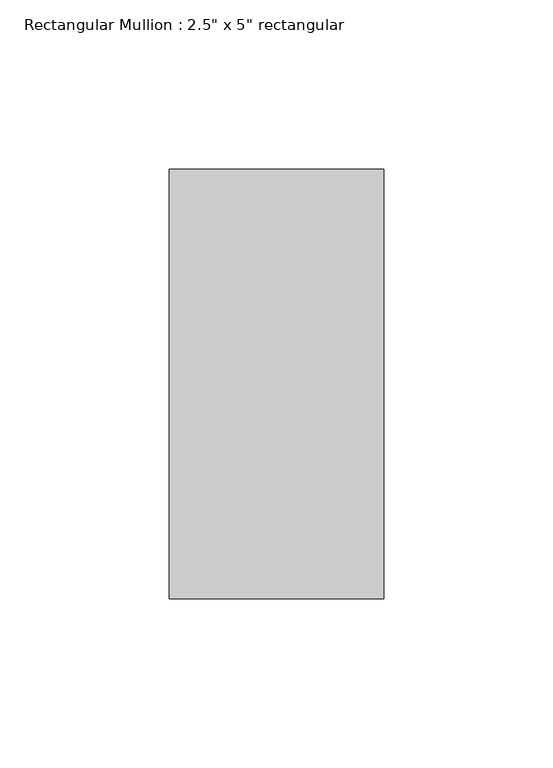
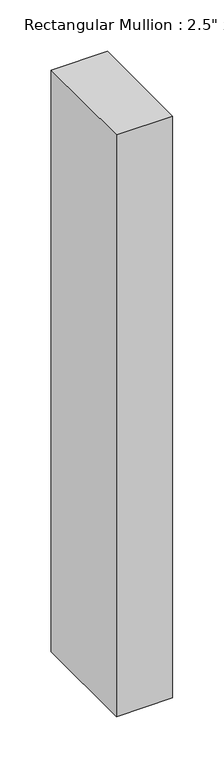
"""IFC4 building model written with IfcOpenShell, lengths in millimetres: member geometry."""

from ifc_helpers import new_model, si_unit, frame, origin, place, context, project, spatial, polyline, outline, extrude, source, transform, mapped, element, save


def member_dcca090c(model_context):
    return source(origin(), model_context, "Body", "SweptSolid", [
        extrude(outline(polyline([(0.0, 63.5), (0.0, -63.5), (-63.5, -63.5), (-63.5, 63.5), (0.0, 63.5)])), frame((0.0, 0.0, -691.9460373), z_axis=(0.0, 0.0, 1.0), x_axis=(1.0, 0.0, 0.0)), (0.0, 0.0, 1.0), 691.9460373),
    ])


if __name__ == "__main__":
    model = new_model("IFC4")
    model_context = context("Model", 3, world=origin())
    ifc_project = project(units=[si_unit("LENGTHUNIT", "METRE", prefix="MILLI")], contexts=[model_context])
    site = spatial("IfcSite", under=ifc_project)
    building = spatial("IfcBuilding", under=site)
    placement = place(None, origin())
    member_shape = member_dcca090c(model_context)
    element("IfcMember", 1, ObjectType="Rectangular Mullion : 2.5\" x 5\" rectangular", at=placement, inside=building, context=model_context, shape_type="MappedRepresentation", body=[
        mapped(member_shape, transform((0.0, 0.0, 0.0), x_axis=(1.0, 0.0, 0.0), y_axis=(0.0, 1.0, 0.0), z_axis=(0.0, 0.0, 1.0))),
    ])
    save(model, "model.ifc")

# Revit data of these elements
# Type "Rectangular Mullion : 2.5\" x 5\" rectangular"
#   built-in parameter 1007304 = 0.416667 (stored number, unit not read)
#   built-in parameter 1007301 = 0.104167 (stored number, unit not read)
#   built-in parameter 1007300 = 0.104167 (stored number, unit not read)
# Element 1 (IfcMember, "Rectangular Mullion : 2.5\" x 5\" rectangular")
#   Materials on its faces: "Aluminum"
# Materials
#   "Aluminum": class "Metal", colour RGB 247 247 247, transparency 0, Description = "Aluminum 6061", Cost = 0
